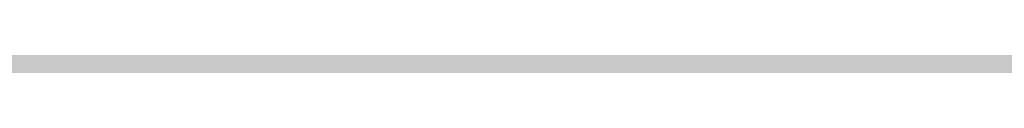
# Model space of a CAD drawing. Units: millimetres. Extents: x 0 to 2267, y 0 to 1823.
# Tile 221 of 256: x 1841.442 to 1842.748, y 1127.419 to 1127.423. Entities that reach past the tile are written whole.
import ezdxf

# ---------------------------------------------------------------- set-up
doc = ezdxf.new("R2010")
doc.units = ezdxf.units.MM
doc.header["$MEASUREMENT"] = 0
doc.layers.add('M-HATC', color=252, linetype='Continuous', lineweight=18)

msp = doc.modelspace()

# ---------------------------------------------------------------- hatches: boundary and pattern name
at = {"layer": 'M-HATC'}
h = msp.add_hatch(color=256, dxfattribs=at)
h.dxf.hatch_style = 1
h.paths.add_polyline_path([(2055.771, 1603.062), (1381.0868, 1603.062), (1381.0868, 1598.062), (2055.771, 1598.062)])
h.paths.add_polyline_path([(2055.771, 1598.062), (1381.0868, 1598.062), (1381.0868, 1593.062), (2055.771, 1593.062)])
h.paths.add_polyline_path([(2051.3074, 1536.7609), (1385.5504, 1536.7609), (1385.5504, 1526.7609), (1387.5504, 1526.7609), (1388.5366, 1525.0528), (1385.3319, 1521.2335), (1385.3319, 1521.2226), (2050.2542, 1522.7491), (2048.3212, 1525.0528), (2049.3074, 1526.7609), (2051.3074, 1526.7609)])
edge = h.paths.add_edge_path()
edge.add_arc((1847.5345, 1379.1492), 135, 222.603061, 222.890851, ccw=False)
edge.add_line((1748.1663, 1287.7656), (1683.0921, 1287.7656))
edge.add_arc((1583.7239, 1379.1492), 135, 317.109149, 317.396939, ccw=False)
edge.add_arc((1678.9686, 1290.6707), 5, 222.8909, 317.1091, ccw=False)
edge.add_arc((1774.2133, 1379.1492), 135, 222.603061, 222.890851, ccw=False)
edge.add_line((1674.8451, 1287.7656), (1609.7709, 1287.7656))
edge.add_arc((1510.4027, 1379.1492), 135, 317.109149, 317.396939, ccw=False)
edge.add_arc((1605.6474, 1290.6707), 5, 222.8909, 317.1091, ccw=False)
edge.add_arc((1700.8921, 1379.1492), 135, 222.603061, 222.890851, ccw=False)
edge.add_line((1601.5239, 1287.7656), (1536.4497, 1287.7656))
edge.add_arc((1437.0815, 1379.1492), 135, 317.109149, 317.396939, ccw=False)
edge.add_arc((1532.3262, 1290.6707), 5, 222.8909, 317.1091, ccw=False)
edge.add_arc((1627.5709, 1379.1492), 135, 222.603061, 222.890851, ccw=False)
edge.add_line((1528.2027, 1287.7656), (1505.9289, 1287.7656))
edge.add_spline(control_points=[(1505.9289, 1287.7656), (1504.2622, 1287.7656), (1504.2622, 1282.7656), (1505.9289, 1282.7656)], knot_values=[0, 0, 0, 0, 5, 5, 5, 5], degree=3, periodic=0)
edge.add_line((1505.9289, 1282.7656), (1930.9289, 1282.7656))
edge.add_spline(control_points=[(1930.9289, 1282.7656), (1932.5956, 1282.7656), (1932.5956, 1287.7656), (1930.9289, 1287.7656)], knot_values=[0, 0, 0, 0, 5, 5, 5, 5], degree=3, periodic=0)
edge.add_line((1930.9289, 1287.7656), (1903.0557, 1287.7656))
edge.add_arc((1803.6875, 1379.1492), 135, 317.109149, 317.396939, ccw=False)
edge.add_arc((1898.9322, 1290.6707), 5, 222.8909, 317.1091, ccw=False)
edge.add_arc((1994.1769, 1379.1492), 135, 222.603061, 222.890851, ccw=False)
edge.add_line((1894.8087, 1287.7656), (1829.7345, 1287.7656))
edge.add_arc((1730.3663, 1379.1492), 135, 317.109149, 317.396939, ccw=False)
edge.add_arc((1825.611, 1290.6707), 5, 222.8909, 317.1091, ccw=False)
edge.add_arc((1920.8557, 1379.1492), 135, 222.603061, 222.890851, ccw=False)
edge.add_line((1821.4875, 1287.7656), (1756.4133, 1287.7656))
edge.add_arc((1657.0451, 1379.1492), 135, 317.109149, 317.396939, ccw=False)
edge.add_arc((1752.2898, 1290.6707), 5, 222.8909, 317.1091, ccw=False)
edge = h.paths.add_edge_path()
edge.add_spline(control_points=[(1843.4289, 1227.2475), (1845.0956, 1227.2475), (1845.0956, 1232.2475), (1843.4289, 1232.2475)], knot_values=[0, 0, 0, 0, 5, 5, 5, 5], degree=3, periodic=0)
edge.add_line((1843.4289, 1232.2475), (1593.4289, 1232.2475))
edge.add_spline(control_points=[(1593.4289, 1232.2475), (1591.7622, 1232.2475), (1591.7622, 1227.2475), (1593.4289, 1227.2475)], knot_values=[0, 0, 0, 0, 5, 5, 5, 5], degree=3, periodic=0)
edge.add_line((1593.4289, 1227.2475), (1843.4289, 1227.2475))
h.paths.add_polyline_path([(1905.9289, 1127.4171), (1530.9289, 1127.4171, 0.414214), (1520.9289, 1117.4171), (1530.9289, 1117.4171), (1915.9289, 1117.4171, 0.414214)])
edge = h.paths.add_edge_path()
edge.add_arc((1397.0858, 1498.4078), 12.7299, 90.78215, 190.87871, ccw=False)
edge.add_line((1396.912, 1511.1365), (1428.0097, 1511.3488))
edge.add_line((1428.0097, 1511.3488), (1433.0097, 1511.3488))
edge.add_line((1433.0097, 1511.3488), (1434.439, 1511.3488))
edge.add_arc((1419.474, 1498.0804), 20, 41.561, 74.08211)
edge.add_line((1424.9592, 1517.3135), (1399.9351, 1517.2561))
edge.add_spline(control_points=[(1399.9307, 1517.2561), (1399.884, 1517.2131), (1399.8328, 1517.1689), (1399.7774, 1517.1236)], knot_values=[11.567499, 11.567499, 11.567499, 11.567499, 11.814249, 11.814249, 11.814249, 11.814249], degree=3, periodic=0)
edge.add_spline(control_points=[(1399.6328, 1517.0099), (1399.5831, 1516.9721), (1399.5307, 1516.9338), (1399.4759, 1516.8947)], knot_values=[11.167718, 11.167718, 11.167718, 11.167718, 11.365188, 11.365188, 11.365188, 11.365188], degree=3, periodic=0)
edge.add_spline(control_points=[(1399.3398, 1516.8001), (1399.1514, 1516.6719), (1398.9384, 1516.5377), (1398.704, 1516.3994)], knot_values=[10.376405, 10.376405, 10.376405, 10.376405, 11.00994, 11.00994, 11.00994, 11.00994], degree=3, periodic=0)
edge.add_spline(control_points=[(1398.6572, 1516.3719), (1398.5789, 1516.326), (1398.4983, 1516.2797), (1398.4155, 1516.2331)], knot_values=[10.125175, 10.125175, 10.125175, 10.125175, 10.334406, 10.334406, 10.334406, 10.334406], degree=3, periodic=0)
edge.add_spline(control_points=[(1398.2642, 1516.1487), (1398.196, 1516.1111), (1398.1263, 1516.0732), (1398.0555, 1516.0351)], knot_values=[9.832246, 9.832246, 9.832246, 9.832246, 9.999658, 9.999658, 9.999658, 9.999658], degree=3, periodic=0)
edge.add_spline(control_points=[(1397.9987, 1516.0048), (1397.7312, 1515.8621), (1397.446, 1515.7171), (1397.1466, 1515.5714)], knot_values=[9.161808, 9.161808, 9.161808, 9.161808, 9.787769, 9.787769, 9.787769, 9.787769], degree=3, periodic=0)
edge.add_spline(control_points=[(1397.1466, 1515.5714), (1396.8418, 1515.423), (1396.5222, 1515.274), (1396.1914, 1515.1262)], knot_values=[8.524455, 8.524455, 8.524455, 8.524455, 9.161808, 9.161808, 9.161808, 9.161808], degree=3, periodic=0)
edge.add_spline(control_points=[(1396.0777, 1515.0756), (1395.9854, 1515.0348), (1395.8922, 1514.994), (1395.7983, 1514.9534)], knot_values=[8.275193, 8.275193, 8.275193, 8.275193, 8.451726, 8.451726, 8.451726, 8.451726], degree=3, periodic=0)
edge.add_spline(control_points=[(1395.6018, 1514.8691), (1395.4997, 1514.8257), (1395.3968, 1514.7824), (1395.2932, 1514.7394)], knot_values=[7.962917, 7.962917, 7.962917, 7.962917, 8.152764, 8.152764, 8.152764, 8.152764], degree=3, periodic=0)
edge.add_spline(control_points=[(1395.2116, 1514.7057), (1394.8278, 1514.5475), (1394.4345, 1514.3929), (1394.0364, 1514.2442)], knot_values=[7.21254, 7.21254, 7.21254, 7.21254, 7.913148, 7.913148, 7.913148, 7.913148], degree=3, periodic=0)
edge.add_spline(control_points=[(1394.0364, 1514.2442), (1393.7076, 1514.1214), (1393.3754, 1514.0027), (1393.0427, 1513.8895)], knot_values=[6.633733, 6.633733, 6.633733, 6.633733, 7.21254, 7.21254, 7.21254, 7.21254], degree=3, periodic=0)
edge.add_spline(control_points=[(1392.8214, 1513.815), (1392.7198, 1513.7812), (1392.6181, 1513.7479), (1392.5166, 1513.7152)], knot_values=[6.328796, 6.328796, 6.328796, 6.328796, 6.505493, 6.505493, 6.505493, 6.505493], degree=3, periodic=0)
edge.add_spline(control_points=[(1392.5166, 1513.7152), (1392.3187, 1513.6515), (1392.1212, 1513.59), (1391.9244, 1513.531)], knot_values=[5.984605, 5.984605, 5.984605, 5.984605, 6.328796, 6.328796, 6.328796, 6.328796], degree=3, periodic=0)
edge.add_spline(control_points=[(1391.7915, 1513.4915), (1391.3122, 1513.3501), (1390.8384, 1513.2239), (1390.3784, 1513.1171)], knot_values=[5.066697, 5.066697, 5.066697, 5.066697, 5.907055, 5.907055, 5.907055, 5.907055], degree=3, periodic=0)
edge.add_spline(control_points=[(1390.3784, 1513.1171), (1390.1797, 1513.071), (1389.9836, 1513.0284), (1389.7907, 1512.9899)], knot_values=[4.70367, 4.70367, 4.70367, 4.70367, 5.066695, 5.066695, 5.066695, 5.066695], degree=3, periodic=0)
edge.add_spline(control_points=[(1389.422, 1512.9204), (1389.2459, 1512.8892), (1389.0729, 1512.8617), (1388.9036, 1512.8381)], knot_values=[4.130571, 4.130571, 4.130571, 4.130571, 4.469816, 4.469816, 4.469816, 4.469816], degree=3, periodic=0)
edge.add_spline(control_points=[(1388.9036, 1512.8381), (1388.591, 1512.7946), (1388.2911, 1512.7644), (1388.0071, 1512.7494)], knot_values=[3.504031, 3.504031, 3.504031, 3.504031, 4.130571, 4.130571, 4.130571, 4.130571], degree=3, periodic=0)
edge.add_spline(control_points=[(1387.9356, 1512.7459), (1387.8538, 1512.7423), (1387.7733, 1512.74), (1387.6944, 1512.739)], knot_values=[3.268866, 3.268866, 3.268866, 3.268866, 3.451164, 3.451164, 3.451164, 3.451164], degree=3, periodic=0)
edge.add_spline(control_points=[(1387.3351, 1512.7443), (1387.2076, 1512.7499), (1387.0847, 1512.7597), (1386.967, 1512.7739)], knot_values=[2.670686, 2.670686, 2.670686, 2.670686, 2.984, 2.984, 2.984, 2.984], degree=3, periodic=0)
edge.add_spline(control_points=[(1386.8327, 1512.7922), (1386.8209, 1512.7941), (1386.8092, 1512.7959), (1386.7975, 1512.7979)], knot_values=[2.516981, 2.516981, 2.516981, 2.516981, 2.549528, 2.549528, 2.549528, 2.549528], degree=3, periodic=0)
edge.add_spline(control_points=[(1386.4526, 1512.8735), (1386.4257, 1512.881), (1386.3993, 1512.889), (1386.3733, 1512.8972)], knot_values=[2.095869, 2.095869, 2.095869, 2.095869, 2.17941, 2.17941, 2.17941, 2.17941], degree=3, periodic=0)
edge.add_spline(control_points=[(1386.0691, 1513.0189), (1386.0634, 1513.0217), (1386.0577, 1513.0246), (1386.052, 1513.0275)], knot_values=[1.72453, 1.72453, 1.72453, 1.72453, 1.745933, 1.745933, 1.745933, 1.745933], degree=3, periodic=0)
edge.add_arc((1399.474, 1498.0804), 20, 131.82432, 180)
edge.add_arc((1630.3336, 1505.5484), 250.9708, 181.705176, 236.427975)
edge.add_arc((1605.3399, 1483.3044), 218.7822, 238.660829, 243.34961)
edge.add_arc((1647.0911, 1510.3592), 262.8986, 183.129836, 237.853442, ccw=False)
h.paths.add_polyline_path([(1406.5369, 1391.9644, 0.149382), (1491.5506, 1296.4418, -0.129517)], flags=17)
edge = h.paths.add_edge_path()
edge.add_arc((2037.3838, 1498.0804), 20, 0, 48.26587)
edge.add_spline(control_points=[(2050.6973, 1513.0052), (2050.6512, 1512.9847), (2050.6034, 1512.9655), (2050.5539, 1512.9477)], knot_values=[1.835652, 1.835652, 1.835652, 1.835652, 2.000781, 2.000781, 2.000781, 2.000781], degree=3, periodic=0)
edge.add_spline(control_points=[(2050.4616, 1512.9166), (2050.479, 1512.9221), (2050.4963, 1512.9277), (2050.5133, 1512.9335)], knot_values=[2.045477, 2.045477, 2.045477, 2.045477, 2.101389, 2.101389, 2.101389, 2.101389], degree=3, periodic=0)
edge.add_spline(control_points=[(2050.129, 1512.8342), (2050.1984, 1512.8473), (2050.2657, 1512.8623), (2050.3308, 1512.8792)], knot_values=[2.237629, 2.237629, 2.237629, 2.237629, 2.435841, 2.435841, 2.435841, 2.435841], degree=3, periodic=0)
edge.add_spline(control_points=[(2050.0946, 1512.8278), (2050.1061, 1512.8299), (2050.1176, 1512.832), (2050.129, 1512.8342)], knot_values=[2.435841, 2.435841, 2.435841, 2.435841, 2.468321, 2.468321, 2.468321, 2.468321], degree=3, periodic=0)
edge.add_spline(control_points=[(2049.7843, 1512.7851), (2049.8552, 1512.7922), (2049.9243, 1512.8008), (2049.9917, 1512.8109)], knot_values=[2.563852, 2.563852, 2.563852, 2.563852, 2.748541, 2.748541, 2.748541, 2.748541], degree=3, periodic=0)
edge.add_spline(control_points=[(2049.4052, 1512.7617), (2049.5364, 1512.7653), (2049.6629, 1512.773), (2049.7843, 1512.7851)], knot_values=[2.748541, 2.748541, 2.748541, 2.748541, 3.064882, 3.064882, 3.064882, 3.064882], degree=3, periodic=0)
edge.add_spline(control_points=[(2049.1698, 1512.7597), (2049.2336, 1512.7591), (2049.2965, 1512.7594), (2049.3584, 1512.7606)], knot_values=[3.102309, 3.102309, 3.102309, 3.102309, 3.2503, 3.2503, 3.2503, 3.2503], degree=3, periodic=0)
edge.add_spline(control_points=[(2048.8573, 1512.7691), (2048.9638, 1512.7638), (2049.068, 1512.7606), (2049.1698, 1512.7597)], knot_values=[3.2503, 3.2503, 3.2503, 3.2503, 3.486069, 3.486069, 3.486069, 3.486069], degree=3, periodic=0)
edge.add_spline(control_points=[(2048.6924, 1512.7789), (2048.3729, 1512.8009), (2048.0345, 1512.8411), (2047.6817, 1512.897)], knot_values=[3.606429, 3.606429, 3.606429, 3.606429, 4.2989, 4.2989, 4.2989, 4.2989], degree=3, periodic=0)
edge.add_spline(control_points=[(2047.6817, 1512.897), (2047.5458, 1512.9185), (2047.4077, 1512.9424), (2047.2678, 1512.9685)], knot_values=[4.2989, 4.2989, 4.2989, 4.2989, 4.565769, 4.565769, 4.565769, 4.565769], degree=3, periodic=0)
edge.add_spline(control_points=[(2047.2678, 1512.9685), (2047.1449, 1512.9914), (2047.0207, 1513.016), (2046.8951, 1513.0422)], knot_values=[4.565769, 4.565769, 4.565769, 4.565769, 4.799971, 4.799971, 4.799971, 4.799971], degree=3, periodic=0)
edge.add_spline(control_points=[(2046.8951, 1513.0422), (2046.5286, 1513.1188), (2046.1513, 1513.209), (2045.7676, 1513.3107)], knot_values=[4.799971, 4.799971, 4.799971, 4.799971, 5.483718, 5.483718, 5.483718, 5.483718], degree=3, periodic=0)
edge.add_spline(control_points=[(2045.7676, 1513.3107), (2045.3724, 1513.4154), (2044.9704, 1513.5322), (2044.5662, 1513.6588)], knot_values=[5.483718, 5.483718, 5.483718, 5.483718, 6.187866, 6.187866, 6.187866, 6.187866], degree=3, periodic=0)
edge.add_spline(control_points=[(2044.5662, 1513.6588), (2044.4149, 1513.7061), (2044.2633, 1513.7549), (2044.1116, 1513.8048)], knot_values=[6.187866, 6.187866, 6.187866, 6.187866, 6.451551, 6.451551, 6.451551, 6.451551], degree=3, periodic=0)
edge.add_spline(control_points=[(2044.1116, 1513.8048), (2043.9967, 1513.8427), (2043.8817, 1513.8813), (2043.7668, 1513.9205)], knot_values=[6.451551, 6.451551, 6.451551, 6.451551, 6.651434, 6.651434, 6.651434, 6.651434], degree=3, periodic=0)
edge.add_spline(control_points=[(2043.7668, 1513.9205), (2043.3716, 1514.0554), (2042.9774, 1514.1979), (2042.5886, 1514.3458)], knot_values=[6.651434, 6.651434, 6.651434, 6.651434, 7.338879, 7.338879, 7.338879, 7.338879], degree=3, periodic=0)
edge.add_spline(control_points=[(2042.5886, 1514.3458), (2042.1643, 1514.5071), (2041.7465, 1514.6749), (2041.3409, 1514.846)], knot_values=[7.338879, 7.338879, 7.338879, 7.338879, 8.089209, 8.089209, 8.089209, 8.089209], degree=3, periodic=0)
edge.add_spline(control_points=[(2041.3409, 1514.846), (2041.1028, 1514.9465), (2040.869, 1515.0481), (2040.6405, 1515.1502)], knot_values=[8.089209, 8.089209, 8.089209, 8.089209, 8.529587, 8.529587, 8.529587, 8.529587], degree=3, periodic=0)
edge.add_spline(control_points=[(2040.51, 1515.2089), (2040.0824, 1515.4022), (2039.6747, 1515.5971), (2039.295, 1515.7894)], knot_values=[8.613818, 8.613818, 8.613818, 8.613818, 9.44571, 9.44571, 9.44571, 9.44571], degree=3, periodic=0)
edge.add_spline(control_points=[(2039.295, 1515.7894), (2039.0618, 1515.9075), (2038.8391, 1516.0246), (2038.6288, 1516.1398)], knot_values=[9.44571, 9.44571, 9.44571, 9.44571, 9.956404, 9.956404, 9.956404, 9.956404], degree=3, periodic=0)
edge.add_spline(control_points=[(2038.6288, 1516.1398), (2038.5187, 1516.2001), (2038.4121, 1516.2598), (2038.309, 1516.3189)], knot_values=[9.956404, 9.956404, 9.956404, 9.956404, 10.223542, 10.223542, 10.223542, 10.223542], degree=3, periodic=0)
edge.add_spline(control_points=[(2038.309, 1516.3189), (2038.2138, 1516.3735), (2038.1216, 1516.4276), (2038.0328, 1516.481)], knot_values=[10.223542, 10.223542, 10.223542, 10.223542, 10.47051, 10.47051, 10.47051, 10.47051], degree=3, periodic=0)
edge.add_spline(control_points=[(2038.0328, 1516.481), (2037.7855, 1516.6296), (2037.5639, 1516.773), (2037.3722, 1516.909)], knot_values=[10.47051, 10.47051, 10.47051, 10.47051, 11.15767, 11.15767, 11.15767, 11.15767], degree=3, periodic=0)
edge.add_spline(control_points=[(2037.3722, 1516.909), (2037.2789, 1516.9752), (2037.1927, 1517.0396), (2037.1142, 1517.102)], knot_values=[11.15767, 11.15767, 11.15767, 11.15767, 11.49227, 11.49227, 11.49227, 11.49227], degree=3, periodic=0)
edge.add_spline(control_points=[(2036.8564, 1517.3259), (2036.9148, 1517.2692), (2036.9814, 1517.2103), (2037.0557, 1517.1492)], knot_values=[11.577341, 11.577341, 11.577341, 11.577341, 11.91035, 11.91035, 11.91035, 11.91035], degree=3, periodic=0)
edge.add_spline(control_points=[(2036.8074, 1517.3748), (2036.823, 1517.3587), (2036.8393, 1517.3424), (2036.8564, 1517.3259)], knot_values=[11.91035, 11.91035, 11.91035, 11.91035, 12.007402, 12.007402, 12.007402, 12.007402], degree=3, periodic=0)
edge.add_spline(control_points=[(2036.7017, 1517.494), (2036.7104, 1517.483), (2036.7196, 1517.4719), (2036.7291, 1517.4606)], knot_values=[12.184155, 12.184155, 12.184155, 12.184155, 12.255409, 12.255409, 12.255409, 12.255409], degree=3, periodic=0)
edge.add_spline(control_points=[(2036.6159, 1517.6205), (2036.62, 1517.613), (2036.6243, 1517.6055), (2036.6289, 1517.5979)], knot_values=[12.487913, 12.487913, 12.487913, 12.487913, 12.541035, 12.541035, 12.541035, 12.541035], degree=3, periodic=0)
edge.add_spline(control_points=[(2036.5635, 1517.786), (2036.5637, 1517.7794), (2036.5642, 1517.7726), (2036.565, 1517.7658)], knot_values=[12.911761, 12.911761, 12.911761, 12.911761, 12.968286, 12.968286, 12.968286, 12.968286], degree=3, periodic=0)
edge.add_spline(control_points=[(2036.6166, 1517.9304), (2036.6125, 1517.9259), (2036.6086, 1517.9212), (2036.6049, 1517.9165)], knot_values=[13.382527, 13.382527, 13.382527, 13.382527, 13.433791, 13.433791, 13.433791, 13.433791], degree=3, periodic=0)
edge.add_spline(control_points=[(2036.749, 1518.017), (2036.7361, 1518.0116), (2036.7239, 1518.006), (2036.7124, 1518.0002)], knot_values=[13.726299, 13.726299, 13.726299, 13.726299, 13.809928, 13.809928, 13.809928, 13.809928], degree=3, periodic=0)
edge.add_spline(control_points=[(2036.8604, 1518.0528), (2036.8386, 1518.0474), (2036.8181, 1518.0416), (2036.7988, 1518.0353)], knot_values=[13.910887, 13.910887, 13.910887, 13.910887, 14.02153, 14.02153, 14.02153, 14.02153], degree=3, periodic=0)
edge.add_line((2036.9639, 1518.0804), (2032.3838, 1518.0804))
edge.add_line((2032.3838, 1518.0804), (2027.3838, 1518.0804))
edge.add_line((2027.3838, 1518.0804), (2022.3838, 1518.0804))
edge.add_line((2022.3838, 1518.0804), (2017.3838, 1518.0804))
edge.add_arc((2017.3838, 1498.0804), 20, 90, 138.439)
edge.add_line((2002.4188, 1511.3488), (2003.8481, 1511.3488))
edge.add_line((2003.8481, 1511.3488), (2008.8481, 1511.3488))
edge.add_line((2008.8481, 1511.3488), (2039.772, 1511.1377))
edge.add_arc((2039.772, 1498.4078), 12.7299, -10.87871, 90, ccw=False)
edge.add_arc((1789.7668, 1510.3592), 262.8986, 302.146558, 356.870164, ccw=False)
edge.add_arc((1831.5179, 1483.3044), 218.7822, 296.65039, 301.339171)
edge.add_arc((1806.5242, 1505.5484), 250.9708, 303.572025, 358.294824)
h.paths.add_polyline_path([(2030.321, 1391.9644, -0.129517), (1945.3072, 1296.4418, 0.149382)], flags=17)
edge = h.paths.add_edge_path()
edge.add_spline(control_points=[(2037.2464, 1518.0821), (2037.2898, 1518.081), (2037.3355, 1518.0804), (2037.3838, 1518.0804)], knot_values=[0.000012, 0.000012, 0.000012, 0.000012, 0.144754, 0.144754, 0.144754, 0.144754], degree=3, periodic=0)
edge.add_line((2037.3357, 1518.0804), (2037.0096, 1518.0804))
edge.add_spline(control_points=[(2037.0096, 1518.0804), (2036.9822, 1518.0768), (2036.956, 1518.0727), (2036.9312, 1518.0681)], knot_values=[14.13465, 14.13465, 14.13465, 14.13465, 14.247197, 14.247197, 14.247197, 14.247197], degree=3, periodic=0)
edge.add_spline(control_points=[(2036.9312, 1518.0681), (2036.9276, 1518.0674), (2036.9241, 1518.0667), (2036.9205, 1518.0661)], knot_values=[14.118315, 14.118315, 14.118315, 14.118315, 14.13465, 14.13465, 14.13465, 14.13465], degree=3, periodic=0)
edge.add_spline(control_points=[(2036.9205, 1518.0661), (2036.9118, 1518.0644), (2036.9032, 1518.0626), (2036.8948, 1518.0608)], knot_values=[14.078086, 14.078086, 14.078086, 14.078086, 14.118315, 14.118315, 14.118315, 14.118315], degree=3, periodic=0)
edge.add_spline(control_points=[(2036.8948, 1518.0608), (2036.883, 1518.0583), (2036.8716, 1518.0556), (2036.8604, 1518.0528)], knot_values=[14.02153, 14.02153, 14.02153, 14.02153, 14.078086, 14.078086, 14.078086, 14.078086], degree=3, periodic=0)
edge.add_spline(control_points=[(2036.8604, 1518.0528), (2036.8386, 1518.0474), (2036.8181, 1518.0416), (2036.7988, 1518.0353)], knot_values=[13.910887, 13.910887, 13.910887, 13.910887, 14.02153, 14.02153, 14.02153, 14.02153], degree=3, periodic=0)
edge.add_spline(control_points=[(2036.7988, 1518.0353), (2036.7981, 1518.035), (2036.7974, 1518.0348), (2036.7967, 1518.0346)], knot_values=[13.906906, 13.906906, 13.906906, 13.906906, 13.910887, 13.910887, 13.910887, 13.910887], degree=3, periodic=0)
edge.add_spline(control_points=[(2036.7967, 1518.0346), (2036.7882, 1518.0318), (2036.7799, 1518.0289), (2036.7719, 1518.0259)], knot_values=[13.857826, 13.857826, 13.857826, 13.857826, 13.906906, 13.906906, 13.906906, 13.906906], degree=3, periodic=0)
edge.add_spline(control_points=[(2036.7719, 1518.0259), (2036.764, 1518.023), (2036.7564, 1518.02), (2036.749, 1518.017)], knot_values=[13.809928, 13.809928, 13.809928, 13.809928, 13.857826, 13.857826, 13.857826, 13.857826], degree=3, periodic=0)
edge.add_spline(control_points=[(2036.749, 1518.017), (2036.7361, 1518.0116), (2036.7239, 1518.006), (2036.7124, 1518.0002)], knot_values=[13.726299, 13.726299, 13.726299, 13.726299, 13.809928, 13.809928, 13.809928, 13.809928], degree=3, periodic=0)
edge.add_spline(control_points=[(2036.7124, 1518.0002), (2036.7121, 1518), (2036.7118, 1517.9999), (2036.7115, 1517.9997)], knot_values=[13.723993, 13.723993, 13.723993, 13.723993, 13.726299, 13.726299, 13.726299, 13.726299], degree=3, periodic=0)
edge.add_spline(control_points=[(2036.7115, 1517.9997), (2036.7063, 1517.9971), (2036.7013, 1517.9944), (2036.6965, 1517.9917)], knot_values=[13.686536, 13.686536, 13.686536, 13.686536, 13.723993, 13.723993, 13.723993, 13.723993], degree=3, periodic=0)
edge.add_spline(control_points=[(2036.6965, 1517.9917), (2036.6919, 1517.9891), (2036.6874, 1517.9865), (2036.6831, 1517.9839)], knot_values=[13.651251, 13.651251, 13.651251, 13.651251, 13.686536, 13.686536, 13.686536, 13.686536], degree=3, periodic=0)
edge.add_spline(control_points=[(2036.6831, 1517.9839), (2036.6764, 1517.9798), (2036.67, 1517.9757), (2036.6639, 1517.9714)], knot_values=[13.596804, 13.596804, 13.596804, 13.596804, 13.651251, 13.651251, 13.651251, 13.651251], degree=3, periodic=0)
edge.add_spline(control_points=[(2036.6639, 1517.9714), (2036.6636, 1517.9712), (2036.6633, 1517.9709), (2036.6629, 1517.9707)], knot_values=[13.593956, 13.593956, 13.593956, 13.593956, 13.596804, 13.596804, 13.596804, 13.596804], degree=3, periodic=0)
edge.add_spline(control_points=[(2036.6629, 1517.9707), (2036.6603, 1517.9689), (2036.6577, 1517.967), (2036.6552, 1517.9651)], knot_values=[13.570322, 13.570322, 13.570322, 13.570322, 13.593956, 13.593956, 13.593956, 13.593956], degree=3, periodic=0)
edge.add_spline(control_points=[(2036.6552, 1517.9651), (2036.6525, 1517.9631), (2036.6499, 1517.9611), (2036.6474, 1517.9591)], knot_values=[13.545477, 13.545477, 13.545477, 13.545477, 13.570322, 13.570322, 13.570322, 13.570322], degree=3, periodic=0)
edge.add_spline(control_points=[(2036.6474, 1517.9591), (2036.6472, 1517.9589), (2036.6471, 1517.9588), (2036.6469, 1517.9587)], knot_values=[13.543931, 13.543931, 13.543931, 13.543931, 13.545477, 13.545477, 13.545477, 13.545477], degree=3, periodic=0)
edge.add_spline(control_points=[(2036.6469, 1517.9587), (2036.6412, 1517.9541), (2036.6358, 1517.9494), (2036.6307, 1517.9447)], knot_values=[13.488237, 13.488237, 13.488237, 13.488237, 13.543931, 13.543931, 13.543931, 13.543931], degree=3, periodic=0)
edge.add_spline(control_points=[(2036.6307, 1517.9447), (2036.6282, 1517.9423), (2036.6257, 1517.9399), (2036.6233, 1517.9374)], knot_values=[13.460307, 13.460307, 13.460307, 13.460307, 13.488237, 13.488237, 13.488237, 13.488237], degree=3, periodic=0)
edge.add_spline(control_points=[(2036.6233, 1517.9374), (2036.6215, 1517.9356), (2036.6198, 1517.9338), (2036.6181, 1517.932)], knot_values=[13.439712, 13.439712, 13.439712, 13.439712, 13.460307, 13.460307, 13.460307, 13.460307], degree=3, periodic=0)
edge.add_spline(control_points=[(2036.6181, 1517.932), (2036.6176, 1517.9315), (2036.6171, 1517.9309), (2036.6166, 1517.9304)], knot_values=[13.433791, 13.433791, 13.433791, 13.433791, 13.439712, 13.439712, 13.439712, 13.439712], degree=3, periodic=0)
edge.add_spline(control_points=[(2036.6166, 1517.9304), (2036.6125, 1517.9259), (2036.6086, 1517.9212), (2036.6049, 1517.9165)], knot_values=[13.382527, 13.382527, 13.382527, 13.382527, 13.433791, 13.433791, 13.433791, 13.433791], degree=3, periodic=0)
edge.add_spline(control_points=[(2036.6049, 1517.9165), (2036.6026, 1517.9135), (2036.6004, 1517.9104), (2036.5982, 1517.9074)], knot_values=[13.350017, 13.350017, 13.350017, 13.350017, 13.382527, 13.382527, 13.382527, 13.382527], degree=3, periodic=0)
edge.add_spline(control_points=[(2036.5982, 1517.9074), (2036.5972, 1517.9059), (2036.5962, 1517.9043), (2036.5952, 1517.9028)], knot_values=[13.333922, 13.333922, 13.333922, 13.333922, 13.350017, 13.350017, 13.350017, 13.350017], degree=3, periodic=0)
edge.add_spline(control_points=[(2036.5952, 1517.9028), (2036.5945, 1517.9018), (2036.5939, 1517.9009), (2036.5933, 1517.8999)], knot_values=[13.323828, 13.323828, 13.323828, 13.323828, 13.333922, 13.333922, 13.333922, 13.333922], degree=3, periodic=0)
edge.add_spline(control_points=[(2036.5933, 1517.8999), (2036.5905, 1517.8955), (2036.5879, 1517.8909), (2036.5855, 1517.8864)], knot_values=[13.277545, 13.277545, 13.277545, 13.277545, 13.323828, 13.323828, 13.323828, 13.323828], degree=3, periodic=0)
edge.add_spline(control_points=[(2036.5855, 1517.8864), (2036.5836, 1517.8827), (2036.5817, 1517.8789), (2036.5801, 1517.8751)], knot_values=[13.240119, 13.240119, 13.240119, 13.240119, 13.277545, 13.277545, 13.277545, 13.277545], degree=3, periodic=0)
edge.add_spline(control_points=[(2036.5801, 1517.8751), (2036.5795, 1517.8739), (2036.579, 1517.8727), (2036.5785, 1517.8715)], knot_values=[13.228211, 13.228211, 13.228211, 13.228211, 13.240119, 13.240119, 13.240119, 13.240119], degree=3, periodic=0)
edge.add_spline(control_points=[(2036.5785, 1517.8715), (2036.578, 1517.8702), (2036.5774, 1517.869), (2036.5769, 1517.8677)], knot_values=[13.215717, 13.215717, 13.215717, 13.215717, 13.228211, 13.228211, 13.228211, 13.228211], degree=3, periodic=0)
edge.add_spline(control_points=[(2036.5769, 1517.8677), (2036.5755, 1517.864), (2036.5741, 1517.8603), (2036.5729, 1517.8565)], knot_values=[13.179847, 13.179847, 13.179847, 13.179847, 13.215717, 13.215717, 13.215717, 13.215717], degree=3, periodic=0)
edge.add_spline(control_points=[(2036.5729, 1517.8565), (2036.5713, 1517.8515), (2036.5699, 1517.8464), (2036.5687, 1517.8413)], knot_values=[13.132017, 13.132017, 13.132017, 13.132017, 13.179847, 13.179847, 13.179847, 13.179847], degree=3, periodic=0)
edge.add_spline(control_points=[(2036.5687, 1517.8413), (2036.5684, 1517.8402), (2036.5682, 1517.8392), (2036.568, 1517.8382)], knot_values=[13.122482, 13.122482, 13.122482, 13.122482, 13.132017, 13.132017, 13.132017, 13.132017], degree=3, periodic=0)
edge.add_spline(control_points=[(2036.568, 1517.8382), (2036.5676, 1517.8363), (2036.5672, 1517.8345), (2036.5669, 1517.8327)], knot_values=[13.105592, 13.105592, 13.105592, 13.105592, 13.122482, 13.122482, 13.122482, 13.122482], degree=3, periodic=0)
edge.add_spline(control_points=[(2036.5669, 1517.8327), (2036.5662, 1517.8292), (2036.5657, 1517.8257), (2036.5652, 1517.8222)], knot_values=[13.074063, 13.074063, 13.074063, 13.074063, 13.105592, 13.105592, 13.105592, 13.105592], degree=3, periodic=0)
edge.add_spline(control_points=[(2036.5652, 1517.8222), (2036.5652, 1517.8222), (2036.5652, 1517.8222), (2036.5652, 1517.8222)], knot_values=[13.074043, 13.074043, 13.074043, 13.074043, 13.074063, 13.074063, 13.074063, 13.074063], degree=3, periodic=0)
edge.add_spline(control_points=[(2036.5652, 1517.8222), (2036.5644, 1517.8164), (2036.5639, 1517.8106), (2036.5636, 1517.8046)], knot_values=[13.021884, 13.021884, 13.021884, 13.021884, 13.074043, 13.074043, 13.074043, 13.074043], degree=3, periodic=0)
edge.add_spline(control_points=[(2036.5636, 1517.8046), (2036.5636, 1517.804), (2036.5636, 1517.8034), (2036.5635, 1517.8028)], knot_values=[13.01674, 13.01674, 13.01674, 13.01674, 13.021884, 13.021884, 13.021884, 13.021884], degree=3, periodic=0)
edge.add_spline(control_points=[(2036.5635, 1517.8028), (2036.5634, 1517.8005), (2036.5634, 1517.7982), (2036.5634, 1517.7958)], knot_values=[12.996438, 12.996438, 12.996438, 12.996438, 13.01674, 13.01674, 13.01674, 13.01674], degree=3, periodic=0)
edge.add_spline(control_points=[(2036.5634, 1517.7958), (2036.5633, 1517.7926), (2036.5634, 1517.7893), (2036.5635, 1517.786)], knot_values=[12.968286, 12.968286, 12.968286, 12.968286, 12.996438, 12.996438, 12.996438, 12.996438], degree=3, periodic=0)
edge.add_spline(control_points=[(2036.5635, 1517.786), (2036.5637, 1517.7794), (2036.5642, 1517.7726), (2036.565, 1517.7658)], knot_values=[12.911761, 12.911761, 12.911761, 12.911761, 12.968286, 12.968286, 12.968286, 12.968286], degree=3, periodic=0)
edge.add_spline(control_points=[(2036.565, 1517.7658), (2036.565, 1517.7657), (2036.565, 1517.7656), (2036.565, 1517.7656)], knot_values=[12.911017, 12.911017, 12.911017, 12.911017, 12.911761, 12.911761, 12.911761, 12.911761], degree=3, periodic=0)
edge.add_spline(control_points=[(2036.565, 1517.7656), (2036.5654, 1517.7625), (2036.5658, 1517.7593), (2036.5663, 1517.7562)], knot_values=[12.88528, 12.88528, 12.88528, 12.88528, 12.911017, 12.911017, 12.911017, 12.911017], degree=3, periodic=0)
edge.add_spline(control_points=[(2036.5663, 1517.7562), (2036.5667, 1517.7534), (2036.5672, 1517.7506), (2036.5677, 1517.7478)], knot_values=[12.862519, 12.862519, 12.862519, 12.862519, 12.88528, 12.88528, 12.88528, 12.88528], degree=3, periodic=0)
edge.add_spline(control_points=[(2036.5677, 1517.7478), (2036.5678, 1517.7474), (2036.5679, 1517.7469), (2036.568, 1517.7465)], knot_values=[12.858885, 12.858885, 12.858885, 12.858885, 12.862519, 12.862519, 12.862519, 12.862519], degree=3, periodic=0)
edge.add_spline(control_points=[(2036.568, 1517.7465), (2036.5692, 1517.7399), (2036.5707, 1517.7332), (2036.5724, 1517.7264)], knot_values=[12.8053, 12.8053, 12.8053, 12.8053, 12.858885, 12.858885, 12.858885, 12.858885], degree=3, periodic=0)
edge.add_spline(control_points=[(2036.5724, 1517.7264), (2036.5734, 1517.7226), (2036.5745, 1517.7187), (2036.5756, 1517.7149)], knot_values=[12.775176, 12.775176, 12.775176, 12.775176, 12.8053, 12.8053, 12.8053, 12.8053], degree=3, periodic=0)
edge.add_spline(control_points=[(2036.5756, 1517.7149), (2036.5763, 1517.7125), (2036.577, 1517.7102), (2036.5778, 1517.7078)], knot_values=[12.756759, 12.756759, 12.756759, 12.756759, 12.775176, 12.775176, 12.775176, 12.775176], degree=3, periodic=0)
edge.add_spline(control_points=[(2036.5778, 1517.7078), (2036.5781, 1517.7067), (2036.5784, 1517.7057), (2036.5787, 1517.7047)], knot_values=[12.748742, 12.748742, 12.748742, 12.748742, 12.756759, 12.756759, 12.756759, 12.756759], degree=3, periodic=0)
edge.add_spline(control_points=[(2036.5787, 1517.7047), (2036.5808, 1517.6983), (2036.5831, 1517.6919), (2036.5856, 1517.6854)], knot_values=[12.69959, 12.69959, 12.69959, 12.69959, 12.748742, 12.748742, 12.748742, 12.748742], degree=3, periodic=0)
edge.add_spline(control_points=[(2036.5856, 1517.6854), (2036.5876, 1517.68), (2036.5898, 1517.6746), (2036.5921, 1517.6692)], knot_values=[12.659038, 12.659038, 12.659038, 12.659038, 12.69959, 12.69959, 12.69959, 12.69959], degree=3, periodic=0)
edge.add_spline(control_points=[(2036.5921, 1517.6692), (2036.594, 1517.6648), (2036.5959, 1517.6605), (2036.5979, 1517.6561)], knot_values=[12.626806, 12.626806, 12.626806, 12.626806, 12.659038, 12.659038, 12.659038, 12.659038], degree=3, periodic=0)
edge.add_spline(control_points=[(2036.5979, 1517.6561), (2036.5984, 1517.6551), (2036.5989, 1517.6541), (2036.5993, 1517.6531)], knot_values=[12.619394, 12.619394, 12.619394, 12.619394, 12.626806, 12.626806, 12.626806, 12.626806], degree=3, periodic=0)
edge.add_spline(control_points=[(2036.5993, 1517.6531), (2036.6043, 1517.6424), (2036.6099, 1517.6315), (2036.6159, 1517.6205)], knot_values=[12.541039, 12.541039, 12.541039, 12.541039, 12.619394, 12.619394, 12.619394, 12.619394], degree=3, periodic=0)
edge.add_spline(control_points=[(2036.6159, 1517.6205), (2036.6159, 1517.6205), (2036.6159, 1517.6205), (2036.6159, 1517.6205)], knot_values=[12.541035, 12.541035, 12.541035, 12.541035, 12.541039, 12.541039, 12.541039, 12.541039], degree=3, periodic=0)
edge.add_spline(control_points=[(2036.6159, 1517.6205), (2036.62, 1517.613), (2036.6243, 1517.6055), (2036.6289, 1517.5979)], knot_values=[12.487913, 12.487913, 12.487913, 12.487913, 12.541035, 12.541035, 12.541035, 12.541035], degree=3, periodic=0)
edge.add_spline(control_points=[(2036.6289, 1517.5979), (2036.6326, 1517.5916), (2036.6365, 1517.5853), (2036.6406, 1517.5789)], knot_values=[12.443982, 12.443982, 12.443982, 12.443982, 12.487913, 12.487913, 12.487913, 12.487913], degree=3, periodic=0)
edge.add_spline(control_points=[(2036.6406, 1517.5789), (2036.6414, 1517.5776), (2036.6423, 1517.5763), (2036.6431, 1517.5749)], knot_values=[12.434996, 12.434996, 12.434996, 12.434996, 12.443982, 12.443982, 12.443982, 12.443982], degree=3, periodic=0)
edge.add_spline(control_points=[(2036.6431, 1517.5749), (2036.6531, 1517.5596), (2036.6639, 1517.5439), (2036.6756, 1517.528)], knot_values=[12.329647, 12.329647, 12.329647, 12.329647, 12.434996, 12.434996, 12.434996, 12.434996], degree=3, periodic=0)
edge.add_spline(control_points=[(2036.6756, 1517.528), (2036.6839, 1517.5168), (2036.6925, 1517.5055), (2036.7017, 1517.494)], knot_values=[12.255409, 12.255409, 12.255409, 12.255409, 12.329647, 12.329647, 12.329647, 12.329647], degree=3, periodic=0)
edge.add_spline(control_points=[(2036.7017, 1517.494), (2036.7104, 1517.483), (2036.7196, 1517.4719), (2036.7291, 1517.4606)], knot_values=[12.184155, 12.184155, 12.184155, 12.184155, 12.255409, 12.255409, 12.255409, 12.255409], degree=3, periodic=0)
edge.add_spline(control_points=[(2036.7291, 1517.4606), (2036.7436, 1517.4435), (2036.759, 1517.4262), (2036.7753, 1517.4085)], knot_values=[12.075961, 12.075961, 12.075961, 12.075961, 12.184155, 12.184155, 12.184155, 12.184155], degree=3, periodic=0)
edge.add_spline(control_points=[(2036.7753, 1517.4085), (2036.7763, 1517.4075), (2036.7773, 1517.4064), (2036.7783, 1517.4054)], knot_values=[12.069502, 12.069502, 12.069502, 12.069502, 12.075961, 12.075961, 12.075961, 12.075961], degree=3, periodic=0)
edge.add_spline(control_points=[(2036.7783, 1517.4054), (2036.7877, 1517.3953), (2036.7974, 1517.385), (2036.8074, 1517.3748)], knot_values=[12.007402, 12.007402, 12.007402, 12.007402, 12.069502, 12.069502, 12.069502, 12.069502], degree=3, periodic=0)
edge.add_spline(control_points=[(2036.8074, 1517.3748), (2036.823, 1517.3587), (2036.8393, 1517.3424), (2036.8564, 1517.3259)], knot_values=[11.91035, 11.91035, 11.91035, 11.91035, 12.007402, 12.007402, 12.007402, 12.007402], degree=3, periodic=0)
edge.add_spline(control_points=[(2036.8564, 1517.3259), (2036.9148, 1517.2692), (2036.9814, 1517.2103), (2037.0557, 1517.1492)], knot_values=[11.577341, 11.577341, 11.577341, 11.577341, 11.91035, 11.91035, 11.91035, 11.91035], degree=3, periodic=0)
edge.add_spline(control_points=[(2037.0557, 1517.1492), (2037.0747, 1517.1336), (2037.0942, 1517.1179), (2037.1142, 1517.102)], knot_values=[11.49227, 11.49227, 11.49227, 11.49227, 11.577341, 11.577341, 11.577341, 11.577341], degree=3, periodic=0)
edge.add_spline(control_points=[(2037.1142, 1517.102), (2037.1927, 1517.0396), (2037.2789, 1516.9752), (2037.3722, 1516.909)], knot_values=[11.15767, 11.15767, 11.15767, 11.15767, 11.49227, 11.49227, 11.49227, 11.49227], degree=3, periodic=0)
edge.add_spline(control_points=[(2037.3722, 1516.909), (2037.5639, 1516.773), (2037.7855, 1516.6296), (2038.0328, 1516.481)], knot_values=[10.47051, 10.47051, 10.47051, 10.47051, 11.15767, 11.15767, 11.15767, 11.15767], degree=3, periodic=0)
edge.add_spline(control_points=[(2038.0328, 1516.481), (2038.1216, 1516.4276), (2038.2138, 1516.3735), (2038.309, 1516.3189)], knot_values=[10.223542, 10.223542, 10.223542, 10.223542, 10.47051, 10.47051, 10.47051, 10.47051], degree=3, periodic=0)
edge.add_spline(control_points=[(2038.309, 1516.3189), (2038.4121, 1516.2598), (2038.5187, 1516.2001), (2038.6288, 1516.1398)], knot_values=[9.956404, 9.956404, 9.956404, 9.956404, 10.223542, 10.223542, 10.223542, 10.223542], degree=3, periodic=0)
edge.add_spline(control_points=[(2038.6288, 1516.1398), (2038.8391, 1516.0246), (2039.0618, 1515.9075), (2039.295, 1515.7894)], knot_values=[9.44571, 9.44571, 9.44571, 9.44571, 9.956404, 9.956404, 9.956404, 9.956404], degree=3, periodic=0)
edge.add_spline(control_points=[(2039.295, 1515.7894), (2039.6747, 1515.5971), (2040.0824, 1515.4022), (2040.51, 1515.2089)], knot_values=[8.613818, 8.613818, 8.613818, 8.613818, 9.44571, 9.44571, 9.44571, 9.44571], degree=3, periodic=0)
edge.add_spline(control_points=[(2040.51, 1515.2089), (2040.5533, 1515.1893), (2040.5968, 1515.1697), (2040.6405, 1515.1502)], knot_values=[8.529587, 8.529587, 8.529587, 8.529587, 8.613818, 8.613818, 8.613818, 8.613818], degree=3, periodic=0)
edge.add_spline(control_points=[(2040.6405, 1515.1502), (2040.869, 1515.0481), (2041.1028, 1514.9465), (2041.3409, 1514.846)], knot_values=[8.089209, 8.089209, 8.089209, 8.089209, 8.529587, 8.529587, 8.529587, 8.529587], degree=3, periodic=0)
edge.add_spline(control_points=[(2041.3409, 1514.846), (2041.7465, 1514.6749), (2042.1643, 1514.5071), (2042.5886, 1514.3458)], knot_values=[7.338879, 7.338879, 7.338879, 7.338879, 8.089209, 8.089209, 8.089209, 8.089209], degree=3, periodic=0)
edge.add_spline(control_points=[(2042.5886, 1514.3458), (2042.9774, 1514.1979), (2043.3716, 1514.0554), (2043.7668, 1513.9205)], knot_values=[6.651434, 6.651434, 6.651434, 6.651434, 7.338879, 7.338879, 7.338879, 7.338879], degree=3, periodic=0)
edge.add_spline(control_points=[(2043.7668, 1513.9205), (2043.8817, 1513.8813), (2043.9967, 1513.8427), (2044.1116, 1513.8048)], knot_values=[6.451551, 6.451551, 6.451551, 6.451551, 6.651434, 6.651434, 6.651434, 6.651434], degree=3, periodic=0)
edge.add_spline(control_points=[(2044.1116, 1513.8048), (2044.2633, 1513.7549), (2044.4149, 1513.7061), (2044.5662, 1513.6588)], knot_values=[6.187866, 6.187866, 6.187866, 6.187866, 6.451551, 6.451551, 6.451551, 6.451551], degree=3, periodic=0)
edge.add_spline(control_points=[(2044.5662, 1513.6588), (2044.9704, 1513.5322), (2045.3724, 1513.4154), (2045.7676, 1513.3107)], knot_values=[5.483718, 5.483718, 5.483718, 5.483718, 6.187866, 6.187866, 6.187866, 6.187866], degree=3, periodic=0)
edge.add_spline(control_points=[(2045.7676, 1513.3107), (2046.1513, 1513.209), (2046.5286, 1513.1188), (2046.8951, 1513.0422)], knot_values=[4.799971, 4.799971, 4.799971, 4.799971, 5.483718, 5.483718, 5.483718, 5.483718], degree=3, periodic=0)
edge.add_spline(control_points=[(2046.8951, 1513.0422), (2047.0207, 1513.016), (2047.1449, 1512.9914), (2047.2678, 1512.9685)], knot_values=[4.565769, 4.565769, 4.565769, 4.565769, 4.799971, 4.799971, 4.799971, 4.799971], degree=3, periodic=0)
edge.add_spline(control_points=[(2047.2678, 1512.9685), (2047.4077, 1512.9424), (2047.5458, 1512.9185), (2047.6817, 1512.897)], knot_values=[4.2989, 4.2989, 4.2989, 4.2989, 4.565769, 4.565769, 4.565769, 4.565769], degree=3, periodic=0)
edge.add_spline(control_points=[(2047.6817, 1512.897), (2048.0345, 1512.8411), (2048.3729, 1512.8009), (2048.6924, 1512.7789)], knot_values=[3.606429, 3.606429, 3.606429, 3.606429, 4.2989, 4.2989, 4.2989, 4.2989], degree=3, periodic=0)
edge.add_spline(control_points=[(2048.6924, 1512.7789), (2048.7479, 1512.7751), (2048.8029, 1512.7718), (2048.8573, 1512.7691)], knot_values=[3.486069, 3.486069, 3.486069, 3.486069, 3.606429, 3.606429, 3.606429, 3.606429], degree=3, periodic=0)
edge.add_spline(control_points=[(2048.8573, 1512.7691), (2048.9638, 1512.7638), (2049.068, 1512.7606), (2049.1698, 1512.7597)], knot_values=[3.2503, 3.2503, 3.2503, 3.2503, 3.486069, 3.486069, 3.486069, 3.486069], degree=3, periodic=0)
edge.add_spline(control_points=[(2049.1698, 1512.7597), (2049.2336, 1512.7591), (2049.2965, 1512.7594), (2049.3584, 1512.7606)], knot_values=[3.102309, 3.102309, 3.102309, 3.102309, 3.2503, 3.2503, 3.2503, 3.2503], degree=3, periodic=0)
edge.add_spline(control_points=[(2049.3584, 1512.7606), (2049.3741, 1512.7609), (2049.3897, 1512.7613), (2049.4052, 1512.7617)], knot_values=[3.064882, 3.064882, 3.064882, 3.064882, 3.102309, 3.102309, 3.102309, 3.102309], degree=3, periodic=0)
edge.add_spline(control_points=[(2049.4052, 1512.7617), (2049.5364, 1512.7653), (2049.6629, 1512.773), (2049.7843, 1512.7851)], knot_values=[2.748541, 2.748541, 2.748541, 2.748541, 3.064882, 3.064882, 3.064882, 3.064882], degree=3, periodic=0)
edge.add_spline(control_points=[(2049.7843, 1512.7851), (2049.8552, 1512.7922), (2049.9243, 1512.8008), (2049.9917, 1512.8109)], knot_values=[2.563852, 2.563852, 2.563852, 2.563852, 2.748541, 2.748541, 2.748541, 2.748541], degree=3, periodic=0)
edge.add_spline(control_points=[(2049.9917, 1512.8109), (2050.0265, 1512.8161), (2050.0608, 1512.8218), (2050.0946, 1512.8278)], knot_values=[2.468321, 2.468321, 2.468321, 2.468321, 2.563852, 2.563852, 2.563852, 2.563852], degree=3, periodic=0)
edge.add_spline(control_points=[(2050.0946, 1512.8278), (2050.1061, 1512.8299), (2050.1176, 1512.832), (2050.129, 1512.8342)], knot_values=[2.435841, 2.435841, 2.435841, 2.435841, 2.468321, 2.468321, 2.468321, 2.468321], degree=3, periodic=0)
edge.add_spline(control_points=[(2050.129, 1512.8342), (2050.1984, 1512.8473), (2050.2657, 1512.8623), (2050.3308, 1512.8792)], knot_values=[2.237629, 2.237629, 2.237629, 2.237629, 2.435841, 2.435841, 2.435841, 2.435841], degree=3, periodic=0)
edge.add_spline(control_points=[(2050.3308, 1512.8792), (2050.3754, 1512.8908), (2050.4191, 1512.9032), (2050.4616, 1512.9166)], knot_values=[2.101389, 2.101389, 2.101389, 2.101389, 2.237629, 2.237629, 2.237629, 2.237629], degree=3, periodic=0)
edge.add_spline(control_points=[(2050.4616, 1512.9166), (2050.479, 1512.9221), (2050.4963, 1512.9277), (2050.5133, 1512.9335)], knot_values=[2.045477, 2.045477, 2.045477, 2.045477, 2.101389, 2.101389, 2.101389, 2.101389], degree=3, periodic=0)
edge.add_spline(control_points=[(2050.5133, 1512.9335), (2050.527, 1512.9382), (2050.5405, 1512.9429), (2050.5539, 1512.9477)], knot_values=[2.000781, 2.000781, 2.000781, 2.000781, 2.045477, 2.045477, 2.045477, 2.045477], degree=3, periodic=0)
edge.add_spline(control_points=[(2050.5539, 1512.9477), (2050.6034, 1512.9655), (2050.6512, 1512.9847), (2050.6973, 1513.0052)], knot_values=[1.835652, 1.835652, 1.835652, 1.835652, 2.000781, 2.000781, 2.000781, 2.000781], degree=3, periodic=0)
edge.add_arc((2037.3838, 1498.0804), 20, 48.26587, 90.12993)
edge = h.paths.add_edge_path(flags=16)
edge.add_spline(control_points=[(1386.1389, 1512.9859), (1388.92, 1511.7395), (1398.0387, 1515.5187), (1399.9307, 1517.2561)], knot_values=[1.831046, 1.831046, 1.831046, 1.831046, 11.814249, 11.814249, 11.814249, 11.814249], degree=3, periodic=0)
edge.add_line((1399.9307, 1517.2561), (1393.7435, 1517.2419))
edge.add_arc((1399.474, 1498.0804), 20, 106.6501, 131.8173)
h = msp.add_hatch(color=256, dxfattribs=at)
h.dxf.hatch_style = 1
h.paths.add_polyline_path([(2042.8886, 1580.1796), (2055.771, 1593.062), (1381.0868, 1593.062), (1393.9692, 1580.1796), (1374.086, 1560.2964), (2062.7718, 1560.2964)])
h.paths.add_polyline_path([(1843.4289, 1201.3297), (1843.4289, 1227.2475), (1593.4289, 1227.2475), (1593.4289, 1201.3297, -0.228274), (1574.5989, 1162.2346), (1530.9289, 1127.4171), (1905.9289, 1127.4171), (1862.2589, 1162.2346, -0.228274)])

doc.saveas('drawing.dxf')
